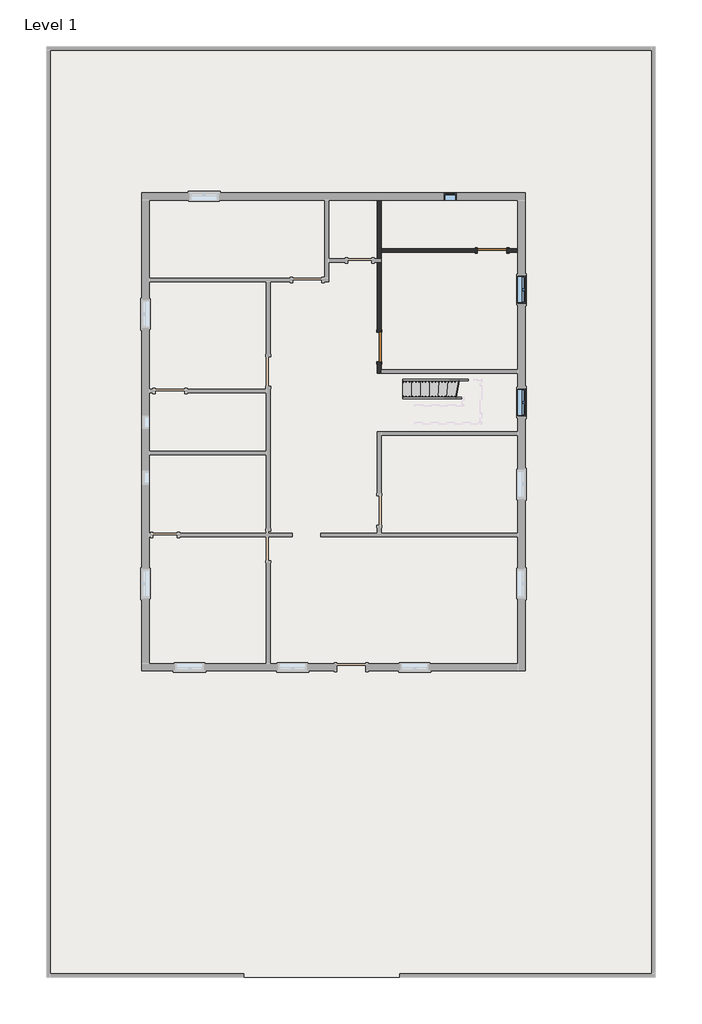
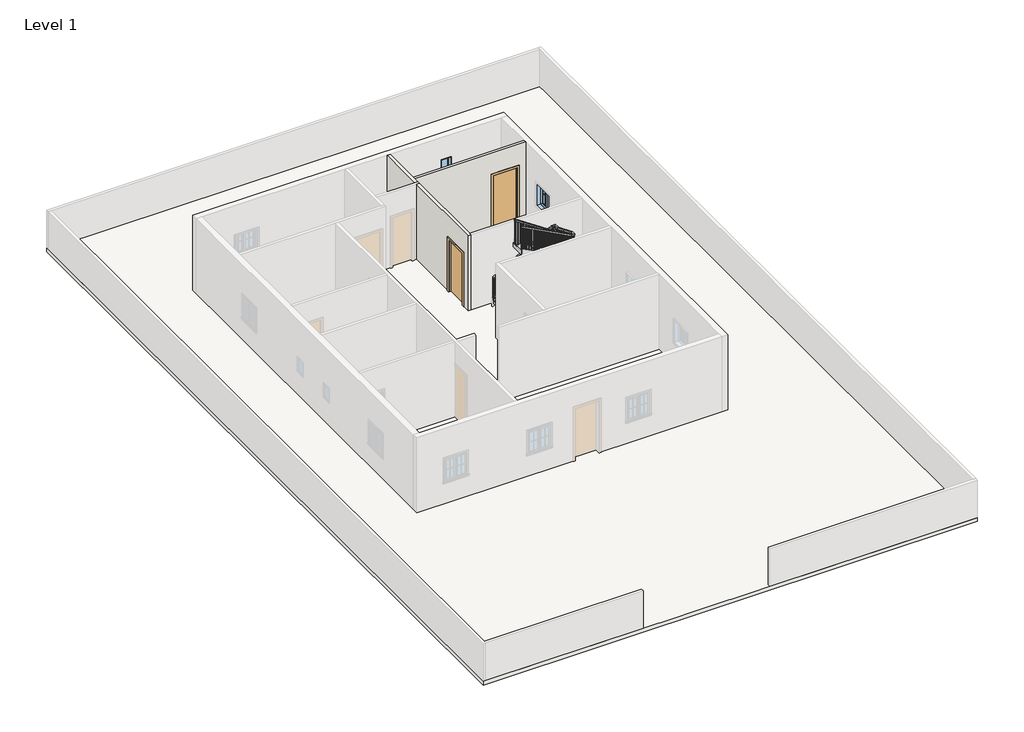
# One storey, part 2 of 3: 3 walls, 3 windows, 2 doors, 2 railings, 1 slab, 1 stair flight.
"""IFC4 building model written with IfcOpenShell, lengths in millimetres."""

from ifc_helpers import new_model, si_unit, frame, origin, place, context, project, spatial, polyline, outline, extrude, faceted_brep, transform, mapped, element, save
from components import door_e5f9f3c4, stair_flight_42adf773, window_373d1f99, window_339605e1

model = new_model("IFC4")

# Units and contexts
model_context = context("Model", 3, world=origin())
ifc_project = project(units=[si_unit("LENGTHUNIT", "METRE", prefix="MILLI")], contexts=[model_context])

# Site, building, storey
site = spatial("IfcSite", under=ifc_project)
building = spatial("IfcBuilding", under=site)
storey = spatial("IfcBuildingStorey", under=building, Name="Level 1", Elevation=0.0)

# Doors
placement = place(None, origin())
door_shape = door_e5f9f3c4(model_context)
element("IfcDoor", 1, ObjectType="Single-Flush : 36\" x 84\"", at=placement, inside=storey, context=model_context, shape_type="MappedRepresentation", body=[
    mapped(door_shape, transform((3624.6756993, 7272.227558, 0.0), x_axis=(1.0, 0.0, 0.0), y_axis=(0.0, 1.0, 0.0), z_axis=(0.0, 0.0, 1.0))),
])
element("IfcDoor", 2, ObjectType="Single-Flush : 36\" x 84\"", at=placement, inside=storey, context=model_context, shape_type="MappedRepresentation", body=[
    mapped(door_shape, transform((100.4256993, 4262.327558, 0.0), x_axis=(0.0, -1.0, 0.0), y_axis=(1.0, 0.0, 0.0), z_axis=(0.0, 0.0, 1.0))),
])

# Railings
element("IfcRailing", 3, ObjectType="Handrail - Rectangular", at=placement, inside=storey, context=model_context, shape_type="SolidModel", body=[
    faceted_brep([(838.4202681, 2744.677558, 1253.0666667), (838.4202681, 2744.677558, 1192.7442501), (838.4202681, 2693.877558, 1192.7442501), (838.4202681, 2693.877558, 1253.0666667), (2663.2073911, 2744.677558, 2421.5510761), (2714.0073911, 2744.677558, 2393.7579377), (2714.0073911, 2693.877558, 2393.7579377), (2663.2073911, 2693.877558, 2421.5510761), (2663.2073911, 2744.677558, 2633.8070819), (2714.0073911, 2744.677558, 2583.0070819), (2714.0073911, 2693.877558, 2583.0070819), (2663.2073911, 2693.877558, 2633.8070819), (2790.2073911, 2744.677558, 2633.8070819), (2790.2073911, 2744.677558, 2583.0070819), (2739.4073911, 2693.877558, 2583.0070819), (2739.4073911, 2693.877558, 2633.8070819), (2790.2073911, 2617.677558, 2633.8070819), (2790.2073911, 2595.5706127, 2583.0070819), (2739.4073911, 2595.5706127, 2583.0070819), (2739.4073911, 2617.677558, 2633.8070819), (2790.2073911, 2490.677558, 2770.1650362), (2790.2073911, 2439.877558, 2750.1723294), (2739.4073911, 2439.877558, 2750.1723294), (2739.4073911, 2490.677558, 2770.1650362), (2790.2073911, 2490.677558, 2985.7137911), (2790.2073911, 2439.877558, 2934.9137911), (2739.4073911, 2439.877558, 2934.9137911), (2739.4073911, 2490.677558, 2985.7137911), (2790.2073911, 2363.677558, 2985.7137911), (2790.2073911, 2363.677558, 2934.9137911), (2739.4073911, 2414.477558, 2934.9137911), (2739.4073911, 2414.477558, 2985.7137911), (2663.2073911, 2363.677558, 2985.7137911), (2647.7076469, 2363.677558, 2934.9137911), (2647.7076469, 2414.477558, 2934.9137911), (2663.2073911, 2414.477558, 2985.7137911), (1211.6756993, 2363.677558, 3962.4), (1211.6756993, 2414.477558, 3962.4), (1211.6756993, 2414.477558, 3901.1707504), (1211.6756993, 2363.677558, 3901.1707504)], [[[0, 1, 2, 3]], [[1, 0, 4, 5]], [[2, 1, 5, 6]], [[3, 2, 6, 7]], [[0, 3, 7, 4]], [[5, 4, 8, 9]], [[6, 5, 9, 10]], [[7, 6, 10, 11]], [[4, 7, 11, 8]], [[9, 8, 12, 13]], [[10, 9, 13, 14]], [[11, 10, 14, 15]], [[8, 11, 15, 12]], [[13, 12, 16, 17]], [[14, 13, 17, 18]], [[15, 14, 18, 19]], [[12, 15, 19, 16]], [[17, 16, 20, 21]], [[18, 17, 21, 22]], [[19, 18, 22, 23]], [[16, 19, 23, 20]], [[21, 20, 24, 25]], [[22, 21, 25, 26]], [[23, 22, 26, 27]], [[20, 23, 27, 24]], [[25, 24, 28, 29]], [[26, 25, 29, 30]], [[27, 26, 30, 31]], [[24, 27, 31, 28]], [[29, 28, 32, 33]], [[30, 29, 33, 34]], [[31, 30, 34, 35]], [[28, 31, 35, 32]], [[36, 37, 38, 39]], [[33, 32, 36, 39]], [[34, 33, 39, 38]], [[35, 34, 38, 37]], [[32, 35, 37, 36]]]),
    extrude(outline(polyline([(3875.1599798, 1250.3323911), (3887.9780756, 1231.2823911), (2878.6666667, 1231.2823911), (2878.6666667, 1250.3323911), (3875.1599798, 1250.3323911)])), frame((0.0, 2379.552558, 0.0), z_axis=(0.0, 1.0, 0.0), x_axis=(0.0, 0.0, 1.0)), (0.0, 0.0, 1.0), 19.05),
    extrude(outline(polyline([(3806.7968022, 1351.9323911), (3819.614898, 1332.8823911), (2878.6666667, 1332.8823911), (2878.6666667, 1351.9323911), (3806.7968022, 1351.9323911)])), frame((0.0, 2379.552558, 0.0), z_axis=(0.0, 1.0, 0.0), x_axis=(0.0, 0.0, 1.0)), (0.0, 0.0, 1.0), 19.05),
    extrude(outline(polyline([(3738.4336246, 1453.5323911), (3751.2517204, 1434.4823911), (2878.6666667, 1434.4823911), (2878.6666667, 1453.5323911), (3738.4336246, 1453.5323911)])), frame((0.0, 2379.552558, 0.0), z_axis=(0.0, 1.0, 0.0), x_axis=(0.0, 0.0, 1.0)), (0.0, 0.0, 1.0), 19.05),
    extrude(outline(polyline([(3670.070447, 1555.1323911), (3682.8885428, 1536.0823911), (2709.3333333, 1536.0823911), (2709.3333333, 1555.1323911), (3670.070447, 1555.1323911)])), frame((0.0, 2379.552558, 0.0), z_axis=(0.0, 1.0, 0.0), x_axis=(0.0, 0.0, 1.0)), (0.0, 0.0, 1.0), 19.05),
    extrude(outline(polyline([(3601.7072694, 1656.7323911), (3614.5253652, 1637.6823911), (2709.3333333, 1637.6823911), (2709.3333333, 1656.7323911), (3601.7072694, 1656.7323911)])), frame((0.0, 2379.552558, 0.0), z_axis=(0.0, 1.0, 0.0), x_axis=(0.0, 0.0, 1.0)), (0.0, 0.0, 1.0), 19.05),
    extrude(outline(polyline([(3533.3440918, 1758.3323911), (3546.1621876, 1739.2823911), (2709.3333333, 1739.2823911), (2709.3333333, 1758.3323911), (3533.3440918, 1758.3323911)])), frame((0.0, 2379.552558, 0.0), z_axis=(0.0, 1.0, 0.0), x_axis=(0.0, 0.0, 1.0)), (0.0, 0.0, 1.0), 19.05),
    extrude(outline(polyline([(3464.9809143, 1859.9323911), (3477.7990101, 1840.8823911), (2540.0, 1840.8823911), (2540.0, 1859.9323911), (3464.9809143, 1859.9323911)])), frame((0.0, 2379.552558, 0.0), z_axis=(0.0, 1.0, 0.0), x_axis=(0.0, 0.0, 1.0)), (0.0, 0.0, 1.0), 19.05),
    extrude(outline(polyline([(3396.6177367, 1961.5323911), (3409.4358325, 1942.4823911), (2540.0, 1942.4823911), (2540.0, 1961.5323911), (3396.6177367, 1961.5323911)])), frame((0.0, 2379.552558, 0.0), z_axis=(0.0, 1.0, 0.0), x_axis=(0.0, 0.0, 1.0)), (0.0, 0.0, 1.0), 19.05),
    extrude(outline(polyline([(3328.2545591, 2063.1323911), (3341.0726549, 2044.0823911), (2370.6666667, 2044.0823911), (2370.6666667, 2063.1323911), (3328.2545591, 2063.1323911)])), frame((0.0, 2379.552558, 0.0), z_axis=(0.0, 1.0, 0.0), x_axis=(0.0, 0.0, 1.0)), (0.0, 0.0, 1.0), 19.05),
    extrude(outline(polyline([(3259.8913815, 2164.7323911), (3272.7094773, 2145.6823911), (2370.6666667, 2145.6823911), (2370.6666667, 2164.7323911), (3259.8913815, 2164.7323911)])), frame((0.0, 2379.552558, 0.0), z_axis=(0.0, 1.0, 0.0), x_axis=(0.0, 0.0, 1.0)), (0.0, 0.0, 1.0), 19.05),
    extrude(outline(polyline([(3191.5282039, 2266.3323911), (3204.3462997, 2247.2823911), (2370.6666667, 2247.2823911), (2370.6666667, 2266.3323911), (3191.5282039, 2266.3323911)])), frame((0.0, 2379.552558, 0.0), z_axis=(0.0, 1.0, 0.0), x_axis=(0.0, 0.0, 1.0)), (0.0, 0.0, 1.0), 19.05),
    extrude(outline(polyline([(3123.1650263, 2367.9323911), (3135.9831221, 2348.8823911), (2201.3333333, 2348.8823911), (2201.3333333, 2367.9323911), (3123.1650263, 2367.9323911)])), frame((0.0, 2379.552558, 0.0), z_axis=(0.0, 1.0, 0.0), x_axis=(0.0, 0.0, 1.0)), (0.0, 0.0, 1.0), 19.05),
    extrude(outline(polyline([(3054.8018487, 2469.5323911), (3067.6199445, 2450.4823911), (2201.3333333, 2450.4823911), (2201.3333333, 2469.5323911), (3054.8018487, 2469.5323911)])), frame((0.0, 2379.552558, 0.0), z_axis=(0.0, 1.0, 0.0), x_axis=(0.0, 0.0, 1.0)), (0.0, 0.0, 1.0), 19.05),
    extrude(outline(polyline([(2986.4386712, 2571.1323911), (2999.256767, 2552.0823911), (2032.0, 2552.0823911), (2032.0, 2571.1323911), (2986.4386712, 2571.1323911)])), frame((0.0, 2379.552558, 0.0), z_axis=(0.0, 1.0, 0.0), x_axis=(0.0, 0.0, 1.0)), (0.0, 0.0, 1.0), 19.05),
    extrude(outline(polyline([(2918.0754936, 2672.7323911), (2930.8935894, 2653.6823911), (2032.0, 2653.6823911), (2032.0, 2672.7323911), (2918.0754936, 2672.7323911)])), frame((0.0, 2379.552558, 0.0), z_axis=(0.0, 1.0, 0.0), x_axis=(0.0, 0.0, 1.0)), (0.0, 0.0, 1.0), 19.05),
    extrude(outline(polyline([(2755.2823911, 2424.002558), (2774.3323911, 2424.002558), (2774.3323911, 2404.952558), (2755.2823911, 2404.952558), (2755.2823911, 2424.002558)])), frame((0.0, 0.0, 1862.6666667), z_axis=(0.0, 0.0, 1.0), x_axis=(1.0, 0.0, 0.0)), (0.0, 0.0, 1.0), 1072.2471245),
    extrude(outline(polyline([(2506.552558, 2678.5844034), (2525.602558, 2658.1307103), (2525.602558, 1693.3333333), (2506.552558, 1693.3333333), (2506.552558, 2678.5844034)])), frame((2755.2823911, 0.0, 0.0), z_axis=(1.0, 0.0, 0.0), x_axis=(0.0, 1.0, 0.0)), (0.0, 0.0, 1.0), 19.05),
    extrude(outline(polyline([(2608.152558, 2569.49804), (2627.202558, 2549.0443468), (2627.202558, 1693.3333333), (2608.152558, 1693.3333333), (2608.152558, 2569.49804)])), frame((2755.2823911, 0.0, 0.0), z_axis=(1.0, 0.0, 0.0), x_axis=(0.0, 1.0, 0.0)), (0.0, 0.0, 1.0), 19.05),
    extrude(outline(polyline([(2657.6952681, 2709.752558), (2657.6952681, 2728.802558), (2676.7452681, 2728.802558), (2676.7452681, 2709.752558), (2657.6952681, 2709.752558)])), frame((0.0, 0.0, 1354.6666667), z_axis=(0.0, 0.0, 1.0), x_axis=(1.0, 0.0, 0.0)), (0.0, 0.0, 1.0), 1228.3404152),
    extrude(outline(polyline([(2304.8389489, 2575.1452681), (2292.6404695, 2556.0952681), (1354.6666667, 2556.0952681), (1354.6666667, 2575.1452681), (2304.8389489, 2575.1452681)])), frame((0.0, 2709.752558, 0.0), z_axis=(0.0, 1.0, 0.0), x_axis=(0.0, 0.0, 1.0)), (0.0, 0.0, 1.0), 19.05),
    extrude(outline(polyline([(2239.7803925, 2473.5452681), (2227.5819131, 2454.4952681), (1185.3333333, 2454.4952681), (1185.3333333, 2473.5452681), (2239.7803925, 2473.5452681)])), frame((0.0, 2709.752558, 0.0), z_axis=(0.0, 1.0, 0.0), x_axis=(0.0, 0.0, 1.0)), (0.0, 0.0, 1.0), 19.05),
    extrude(outline(polyline([(2174.721836, 2371.9452681), (2162.5233567, 2352.8952681), (1185.3333333, 2352.8952681), (1185.3333333, 2371.9452681), (2174.721836, 2371.9452681)])), frame((0.0, 2709.752558, 0.0), z_axis=(0.0, 1.0, 0.0), x_axis=(0.0, 0.0, 1.0)), (0.0, 0.0, 1.0), 19.05),
    extrude(outline(polyline([(2109.6632796, 2270.3452681), (2097.4648003, 2251.2952681), (1185.3333333, 2251.2952681), (1185.3333333, 2270.3452681), (2109.6632796, 2270.3452681)])), frame((0.0, 2709.752558, 0.0), z_axis=(0.0, 1.0, 0.0), x_axis=(0.0, 0.0, 1.0)), (0.0, 0.0, 1.0), 19.05),
    extrude(outline(polyline([(2044.6047232, 2168.7452681), (2032.4062439, 2149.6952681), (1016.0, 2149.6952681), (1016.0, 2168.7452681), (2044.6047232, 2168.7452681)])), frame((0.0, 2709.752558, 0.0), z_axis=(0.0, 1.0, 0.0), x_axis=(0.0, 0.0, 1.0)), (0.0, 0.0, 1.0), 19.05),
    extrude(outline(polyline([(1979.5461668, 2067.1452681), (1967.3476875, 2048.0952681), (1016.0, 2048.0952681), (1016.0, 2067.1452681), (1979.5461668, 2067.1452681)])), frame((0.0, 2709.752558, 0.0), z_axis=(0.0, 1.0, 0.0), x_axis=(0.0, 0.0, 1.0)), (0.0, 0.0, 1.0), 19.05),
    extrude(outline(polyline([(1914.4876104, 1965.5452681), (1902.289131, 1946.4952681), (1016.0, 1946.4952681), (1016.0, 1965.5452681), (1914.4876104, 1965.5452681)])), frame((0.0, 2709.752558, 0.0), z_axis=(0.0, 1.0, 0.0), x_axis=(0.0, 0.0, 1.0)), (0.0, 0.0, 1.0), 19.05),
    extrude(outline(polyline([(1849.4290539, 1863.9452681), (1837.2305746, 1844.8952681), (846.6666667, 1844.8952681), (846.6666667, 1863.9452681), (1849.4290539, 1863.9452681)])), frame((0.0, 2709.752558, 0.0), z_axis=(0.0, 1.0, 0.0), x_axis=(0.0, 0.0, 1.0)), (0.0, 0.0, 1.0), 19.05),
    extrude(outline(polyline([(1784.3704975, 1762.3452681), (1772.1720182, 1743.2952681), (846.6666667, 1743.2952681), (846.6666667, 1762.3452681), (1784.3704975, 1762.3452681)])), frame((0.0, 2709.752558, 0.0), z_axis=(0.0, 1.0, 0.0), x_axis=(0.0, 0.0, 1.0)), (0.0, 0.0, 1.0), 19.05),
    extrude(outline(polyline([(1719.3119411, 1660.7452681), (1707.1134618, 1641.6952681), (677.3333333, 1641.6952681), (677.3333333, 1660.7452681), (1719.3119411, 1660.7452681)])), frame((0.0, 2709.752558, 0.0), z_axis=(0.0, 1.0, 0.0), x_axis=(0.0, 0.0, 1.0)), (0.0, 0.0, 1.0), 19.05),
    extrude(outline(polyline([(1654.2533847, 1559.1452681), (1642.0549054, 1540.0952681), (677.3333333, 1540.0952681), (677.3333333, 1559.1452681), (1654.2533847, 1559.1452681)])), frame((0.0, 2709.752558, 0.0), z_axis=(0.0, 1.0, 0.0), x_axis=(0.0, 0.0, 1.0)), (0.0, 0.0, 1.0), 19.05),
    extrude(outline(polyline([(1589.1948283, 1457.5452681), (1576.9963489, 1438.4952681), (677.3333333, 1438.4952681), (677.3333333, 1457.5452681), (1589.1948283, 1457.5452681)])), frame((0.0, 2709.752558, 0.0), z_axis=(0.0, 1.0, 0.0), x_axis=(0.0, 0.0, 1.0)), (0.0, 0.0, 1.0), 19.05),
    extrude(outline(polyline([(1524.1362719, 1355.9452681), (1511.9377925, 1336.8952681), (508.0, 1336.8952681), (508.0, 1355.9452681), (1524.1362719, 1355.9452681)])), frame((0.0, 2709.752558, 0.0), z_axis=(0.0, 1.0, 0.0), x_axis=(0.0, 0.0, 1.0)), (0.0, 0.0, 1.0), 19.05),
    extrude(outline(polyline([(1459.0777154, 1254.3452681), (1446.8792361, 1235.2952681), (508.0, 1235.2952681), (508.0, 1254.3452681), (1459.0777154, 1254.3452681)])), frame((0.0, 2709.752558, 0.0), z_axis=(0.0, 1.0, 0.0), x_axis=(0.0, 0.0, 1.0)), (0.0, 0.0, 1.0), 19.05),
    extrude(outline(polyline([(1394.019159, 1152.7452681), (1381.8206797, 1133.6952681), (508.0, 1133.6952681), (508.0, 1152.7452681), (1394.019159, 1152.7452681)])), frame((0.0, 2709.752558, 0.0), z_axis=(0.0, 1.0, 0.0), x_axis=(0.0, 0.0, 1.0)), (0.0, 0.0, 1.0), 19.05),
    extrude(outline(polyline([(1328.9606026, 1051.1452681), (1316.7621233, 1032.0952681), (338.6666667, 1032.0952681), (338.6666667, 1051.1452681), (1328.9606026, 1051.1452681)])), frame((0.0, 2709.752558, 0.0), z_axis=(0.0, 1.0, 0.0), x_axis=(0.0, 0.0, 1.0)), (0.0, 0.0, 1.0), 19.05),
    extrude(outline(polyline([(1263.9020462, 949.5452681), (1251.7035669, 930.4952681), (338.6666667, 930.4952681), (338.6666667, 949.5452681), (1263.9020462, 949.5452681)])), frame((0.0, 2709.752558, 0.0), z_axis=(0.0, 1.0, 0.0), x_axis=(0.0, 0.0, 1.0)), (0.0, 0.0, 1.0), 19.05),
    extrude(outline(polyline([(2755.2823911, 2398.602558), (2774.3323911, 2398.602558), (2774.3323911, 2379.552558), (2755.2823911, 2379.552558), (2755.2823911, 2398.602558)])), frame((0.0, 0.0, 1862.6666667), z_axis=(0.0, 0.0, 1.0), x_axis=(1.0, 0.0, 0.0)), (0.0, 0.0, 1.0), 1072.2471245),
    extrude(outline(polyline([(2755.2823911, 2709.752558), (2755.2823911, 2728.802558), (2774.3323911, 2728.802558), (2774.3323911, 2709.752558), (2755.2823911, 2709.752558)])), frame((0.0, 0.0, 1524.0), z_axis=(0.0, 0.0, 1.0), x_axis=(1.0, 0.0, 0.0)), (0.0, 0.0, 1.0), 1059.0070819),
    extrude(outline(polyline([(3888.3526546, 1230.7256993), (3901.1707504, 1211.6756993), (2878.6666667, 1211.6756993), (2878.6666667, 1230.7256993), (3888.3526546, 1230.7256993)])), frame((0.0, 2379.552558, 0.0), z_axis=(0.0, 1.0, 0.0), x_axis=(0.0, 0.0, 1.0)), (0.0, 0.0, 1.0), 19.05),
    extrude(outline(polyline([(1204.9427294, 857.4702681), (1192.7442501, 838.4202681), (338.6666667, 838.4202681), (338.6666667, 857.4702681), (1204.9427294, 857.4702681)])), frame((0.0, 2709.752558, 0.0), z_axis=(0.0, 1.0, 0.0), x_axis=(0.0, 0.0, 1.0)), (0.0, 0.0, 1.0), 19.05),
])
element("IfcRailing", 4, ObjectType="Handrail - Rectangular", at=placement, inside=storey, context=model_context, shape_type="SolidModel", body=[
    faceted_brep([(838.4202681, 3202.4524989, 1253.0666667), (838.4202681, 3202.4524989, 1194.4953096), (838.4202681, 3151.6524989, 1194.4953096), (838.4202681, 3151.6524989, 1253.0666667), (3089.9785641, 3202.4524989, 2545.2368493), (3103.5198636, 3202.4524989, 2494.4368493), (3103.5198636, 3151.6524989, 2494.4368493), (3089.9785641, 3151.6524989, 2545.2368493), (3247.982332, 3202.4524989, 2545.2368493), (3247.982332, 3202.4524989, 2494.4368493), (3197.182332, 3151.6524989, 2494.4368493), (3197.182332, 3151.6524989, 2545.2368493), (3247.982332, 2995.1725832, 2545.2368493), (3247.982332, 2984.9732412, 2494.4368493), (3197.182332, 2984.9732412, 2494.4368493), (3197.182332, 2995.1725832, 2545.2368493), (3247.982332, 2050.6126885, 2940.4552365), (3247.982332, 2040.4133465, 2889.6552365), (3197.182332, 2040.4133465, 2889.6552365), (3197.182332, 2050.6126885, 2940.4552365), (3247.982332, 1905.9026171, 2940.4552365), (3247.982332, 1905.9026171, 2889.6552365), (3197.182332, 1956.7026171, 2889.6552365), (3197.182332, 1956.7026171, 2940.4552365), (3128.9262072, 1905.9026171, 2940.4552365), (3116.2326609, 1905.9026171, 2889.6552365), (3116.2326609, 1956.7026171, 2889.6552365), (3128.9262072, 1956.7026171, 2940.4552365), (1211.6756993, 1905.9026171, 3962.4), (1211.6756993, 1956.7026171, 3962.4), (1211.6756993, 1956.7026171, 3904.8340072), (1211.6756993, 1905.9026171, 3904.8340072)], [[[0, 1, 2, 3]], [[1, 0, 4, 5]], [[2, 1, 5, 6]], [[3, 2, 6, 7]], [[0, 3, 7, 4]], [[5, 4, 8, 9]], [[6, 5, 9, 10]], [[7, 6, 10, 11]], [[4, 7, 11, 8]], [[9, 8, 12, 13]], [[10, 9, 13, 14]], [[11, 10, 14, 15]], [[8, 11, 15, 12]], [[13, 12, 16, 17]], [[14, 13, 17, 18]], [[15, 14, 18, 19]], [[12, 15, 19, 16]], [[17, 16, 20, 21]], [[18, 17, 21, 22]], [[19, 18, 22, 23]], [[16, 19, 23, 20]], [[21, 20, 24, 25]], [[22, 21, 25, 26]], [[23, 22, 26, 27]], [[20, 23, 27, 24]], [[28, 29, 30, 31]], [[25, 24, 28, 31]], [[26, 25, 31, 30]], [[27, 26, 30, 29]], [[24, 27, 29, 28]]]),
    extrude(outline(polyline([(3866.9989368, 1282.657332), (2878.6666667, 1282.657332), (2878.6666667, 1301.707332), (3856.8447876, 1301.707332), (3866.9989368, 1282.657332)])), frame((0.0, 1921.7776171, 0.0), z_axis=(0.0, 1.0, 0.0), x_axis=(0.0, 0.0, 1.0)), (0.0, 0.0, 1.0), 19.05),
    extrude(outline(polyline([(3812.8434743, 1384.257332), (2878.6666667, 1384.257332), (2878.6666667, 1403.307332), (3802.6893251, 1403.307332), (3812.8434743, 1384.257332)])), frame((0.0, 1921.7776171, 0.0), z_axis=(0.0, 1.0, 0.0), x_axis=(0.0, 0.0, 1.0)), (0.0, 0.0, 1.0), 19.05),
    extrude(outline(polyline([(3758.6880118, 1485.857332), (2709.3333333, 1485.857332), (2709.3333333, 1504.907332), (3748.5338626, 1504.907332), (3758.6880118, 1485.857332)])), frame((0.0, 1921.7776171, 0.0), z_axis=(0.0, 1.0, 0.0), x_axis=(0.0, 0.0, 1.0)), (0.0, 0.0, 1.0), 19.05),
    extrude(outline(polyline([(3704.5325493, 1587.457332), (2709.3333333, 1587.457332), (2709.3333333, 1606.507332), (3694.3784001, 1606.507332), (3704.5325493, 1587.457332)])), frame((0.0, 1921.7776171, 0.0), z_axis=(0.0, 1.0, 0.0), x_axis=(0.0, 0.0, 1.0)), (0.0, 0.0, 1.0), 19.05),
    extrude(outline(polyline([(3650.3770868, 1689.057332), (2709.3333333, 1689.057332), (2709.3333333, 1708.107332), (3640.2229376, 1708.107332), (3650.3770868, 1689.057332)])), frame((0.0, 1921.7776171, 0.0), z_axis=(0.0, 1.0, 0.0), x_axis=(0.0, 0.0, 1.0)), (0.0, 0.0, 1.0), 19.05),
    extrude(outline(polyline([(3596.2216243, 1790.657332), (2540.0, 1790.657332), (2540.0, 1809.707332), (3586.0674751, 1809.707332), (3596.2216243, 1790.657332)])), frame((0.0, 1921.7776171, 0.0), z_axis=(0.0, 1.0, 0.0), x_axis=(0.0, 0.0, 1.0)), (0.0, 0.0, 1.0), 19.05),
    extrude(outline(polyline([(3542.0661618, 1892.257332), (2540.0, 1892.257332), (2540.0, 1911.307332), (3531.9120126, 1911.307332), (3542.0661618, 1892.257332)])), frame((0.0, 1921.7776171, 0.0), z_axis=(0.0, 1.0, 0.0), x_axis=(0.0, 0.0, 1.0)), (0.0, 0.0, 1.0), 19.05),
    extrude(outline(polyline([(3487.9106993, 1993.857332), (2540.0, 1993.857332), (2540.0, 2012.907332), (3477.7565501, 2012.907332), (3487.9106993, 1993.857332)])), frame((0.0, 1921.7776171, 0.0), z_axis=(0.0, 1.0, 0.0), x_axis=(0.0, 0.0, 1.0)), (0.0, 0.0, 1.0), 19.05),
    extrude(outline(polyline([(3433.7552369, 2095.457332), (2370.6666667, 2095.457332), (2370.6666667, 2114.507332), (3423.6010876, 2114.507332), (3433.7552369, 2095.457332)])), frame((0.0, 1921.7776171, 0.0), z_axis=(0.0, 1.0, 0.0), x_axis=(0.0, 0.0, 1.0)), (0.0, 0.0, 1.0), 19.05),
    extrude(outline(polyline([(3379.5997744, 2197.057332), (2370.6666667, 2197.057332), (2370.6666667, 2216.107332), (3369.4456251, 2216.107332), (3379.5997744, 2197.057332)])), frame((0.0, 1921.7776171, 0.0), z_axis=(0.0, 1.0, 0.0), x_axis=(0.0, 0.0, 1.0)), (0.0, 0.0, 1.0), 19.05),
    extrude(outline(polyline([(3325.4443119, 2298.657332), (2370.6666667, 2298.657332), (2370.6666667, 2317.707332), (3315.2901626, 2317.707332), (3325.4443119, 2298.657332)])), frame((0.0, 1921.7776171, 0.0), z_axis=(0.0, 1.0, 0.0), x_axis=(0.0, 0.0, 1.0)), (0.0, 0.0, 1.0), 19.05),
    extrude(outline(polyline([(3271.2888494, 2400.257332), (2201.3333333, 2400.257332), (2201.3333333, 2419.307332), (3261.1347002, 2419.307332), (3271.2888494, 2400.257332)])), frame((0.0, 1921.7776171, 0.0), z_axis=(0.0, 1.0, 0.0), x_axis=(0.0, 0.0, 1.0)), (0.0, 0.0, 1.0), 19.05),
    extrude(outline(polyline([(3217.1333869, 2501.857332), (2201.3333333, 2501.857332), (2201.3333333, 2520.907332), (3206.9792377, 2520.907332), (3217.1333869, 2501.857332)])), frame((0.0, 1921.7776171, 0.0), z_axis=(0.0, 1.0, 0.0), x_axis=(0.0, 0.0, 1.0)), (0.0, 0.0, 1.0), 19.05),
    extrude(outline(polyline([(3162.9779244, 2603.457332), (2201.3333333, 2603.457332), (2201.3333333, 2622.507332), (3152.8237752, 2622.507332), (3162.9779244, 2603.457332)])), frame((0.0, 1921.7776171, 0.0), z_axis=(0.0, 1.0, 0.0), x_axis=(0.0, 0.0, 1.0)), (0.0, 0.0, 1.0), 19.05),
    extrude(outline(polyline([(3108.8224619, 2705.057332), (2032.0, 2705.057332), (2032.0, 2724.107332), (3098.6683127, 2724.107332), (3108.8224619, 2705.057332)])), frame((0.0, 1921.7776171, 0.0), z_axis=(0.0, 1.0, 0.0), x_axis=(0.0, 0.0, 1.0)), (0.0, 0.0, 1.0), 19.05),
    extrude(outline(polyline([(3054.6669994, 2806.657332), (2032.0, 2806.657332), (2032.0, 2825.707332), (3044.5128502, 2825.707332), (3054.6669994, 2806.657332)])), frame((0.0, 1921.7776171, 0.0), z_axis=(0.0, 1.0, 0.0), x_axis=(0.0, 0.0, 1.0)), (0.0, 0.0, 1.0), 19.05),
    extrude(outline(polyline([(3000.5115369, 2908.257332), (2032.0, 2908.257332), (2032.0, 2927.307332), (2990.3573877, 2927.307332), (3000.5115369, 2908.257332)])), frame((0.0, 1921.7776171, 0.0), z_axis=(0.0, 1.0, 0.0), x_axis=(0.0, 0.0, 1.0)), (0.0, 0.0, 1.0), 19.05),
    extrude(outline(polyline([(2946.3560744, 3009.857332), (2032.0, 3009.857332), (2032.0, 3028.907332), (2936.2019252, 3028.907332), (2946.3560744, 3009.857332)])), frame((0.0, 1921.7776171, 0.0), z_axis=(0.0, 1.0, 0.0), x_axis=(0.0, 0.0, 1.0)), (0.0, 0.0, 1.0), 19.05),
    extrude(outline(polyline([(2892.2006119, 3111.457332), (1862.6666667, 3111.457332), (1862.6666667, 3130.507332), (2882.0464627, 3130.507332), (2892.2006119, 3111.457332)])), frame((0.0, 1921.7776171, 0.0), z_axis=(0.0, 1.0, 0.0), x_axis=(0.0, 0.0, 1.0)), (0.0, 0.0, 1.0), 19.05),
    extrude(outline(polyline([(3232.107332, 1967.3774989), (3232.107332, 1948.3274989), (3213.057332, 1948.3274989), (3213.057332, 1967.3774989), (3232.107332, 1967.3774989)])), frame((0.0, 0.0, 1862.6666667), z_axis=(0.0, 0.0, 1.0), x_axis=(1.0, 0.0, 0.0)), (0.0, 0.0, 1.0), 1026.9885698),
    extrude(outline(polyline([(2068.9774989, 2877.7035558), (2068.9774989, 1862.6666667), (2049.9274989, 1862.6666667), (2049.9274989, 2885.6743688), (2068.9774989, 2877.7035558)])), frame((3213.057332, 0.0, 0.0), z_axis=(1.0, 0.0, 0.0), x_axis=(0.0, 1.0, 0.0)), (0.0, 0.0, 1.0), 19.05),
    extrude(outline(polyline([(2170.5774989, 2835.1925532), (2170.5774989, 1862.6666667), (2151.5274989, 1862.6666667), (2151.5274989, 2843.1633662), (2170.5774989, 2835.1925532)])), frame((3213.057332, 0.0, 0.0), z_axis=(1.0, 0.0, 0.0), x_axis=(0.0, 1.0, 0.0)), (0.0, 0.0, 1.0), 19.05),
    extrude(outline(polyline([(2272.1774989, 2792.6815506), (2272.1774989, 1862.6666667), (2253.1274989, 1862.6666667), (2253.1274989, 2800.6523636), (2272.1774989, 2792.6815506)])), frame((3213.057332, 0.0, 0.0), z_axis=(1.0, 0.0, 0.0), x_axis=(0.0, 1.0, 0.0)), (0.0, 0.0, 1.0), 19.05),
    extrude(outline(polyline([(2373.7774989, 2750.170548), (2373.7774989, 1862.6666667), (2354.7274989, 1862.6666667), (2354.7274989, 2758.141361), (2373.7774989, 2750.170548)])), frame((3213.057332, 0.0, 0.0), z_axis=(1.0, 0.0, 0.0), x_axis=(0.0, 1.0, 0.0)), (0.0, 0.0, 1.0), 19.05),
    extrude(outline(polyline([(2475.3774989, 2707.6595454), (2475.3774989, 1693.3333333), (2456.3274989, 1693.3333333), (2456.3274989, 2715.6303584), (2475.3774989, 2707.6595454)])), frame((3213.057332, 0.0, 0.0), z_axis=(1.0, 0.0, 0.0), x_axis=(0.0, 1.0, 0.0)), (0.0, 0.0, 1.0), 19.05),
    extrude(outline(polyline([(2576.9774989, 2665.1485428), (2576.9774989, 1693.3333333), (2557.9274989, 1693.3333333), (2557.9274989, 2673.1193558), (2576.9774989, 2665.1485428)])), frame((3213.057332, 0.0, 0.0), z_axis=(1.0, 0.0, 0.0), x_axis=(0.0, 1.0, 0.0)), (0.0, 0.0, 1.0), 19.05),
    extrude(outline(polyline([(2678.5774989, 2622.6375402), (2678.5774989, 1693.3333333), (2659.5274989, 1693.3333333), (2659.5274989, 2630.6083532), (2678.5774989, 2622.6375402)])), frame((3213.057332, 0.0, 0.0), z_axis=(1.0, 0.0, 0.0), x_axis=(0.0, 1.0, 0.0)), (0.0, 0.0, 1.0), 19.05),
    extrude(outline(polyline([(2780.1774989, 2580.1265376), (2780.1774989, 1693.3333333), (2761.1274989, 1693.3333333), (2761.1274989, 2588.0973506), (2780.1774989, 2580.1265376)])), frame((3213.057332, 0.0, 0.0), z_axis=(1.0, 0.0, 0.0), x_axis=(0.0, 1.0, 0.0)), (0.0, 0.0, 1.0), 19.05),
    extrude(outline(polyline([(2881.7774989, 2537.615535), (2881.7774989, 1524.0), (2862.7274989, 1524.0), (2862.7274989, 2545.586348), (2881.7774989, 2537.615535)])), frame((3213.057332, 0.0, 0.0), z_axis=(1.0, 0.0, 0.0), x_axis=(0.0, 1.0, 0.0)), (0.0, 0.0, 1.0), 19.05),
    extrude(outline(polyline([(2983.3774989, 2495.1045324), (2983.3774989, 1524.0), (2964.3274989, 1524.0), (2964.3274989, 2503.0753454), (2983.3774989, 2495.1045324)])), frame((3213.057332, 0.0, 0.0), z_axis=(1.0, 0.0, 0.0), x_axis=(0.0, 1.0, 0.0)), (0.0, 0.0, 1.0), 19.05),
    extrude(outline(polyline([(3232.107332, 3084.9774989), (3232.107332, 3065.9274989), (3213.057332, 3065.9274989), (3213.057332, 3084.9774989), (3232.107332, 3084.9774989)])), frame((0.0, 0.0, 1524.0), z_axis=(0.0, 0.0, 1.0), x_axis=(1.0, 0.0, 0.0)), (0.0, 0.0, 1.0), 970.4368493),
    extrude(outline(polyline([(3165.6952681, 3186.5774989), (3184.7452681, 3186.5774989), (3184.7452681, 3167.5274989), (3165.6952681, 3167.5274989), (3165.6952681, 3186.5774989)])), frame((0.0, 0.0, 1524.0), z_axis=(0.0, 0.0, 1.0), x_axis=(1.0, 0.0, 0.0)), (0.0, 0.0, 1.0), 970.4368493),
    extrude(outline(polyline([(2471.8110585, 3064.0952681), (1524.0, 3064.0952681), (1524.0, 3083.1452681), (2482.743861, 3083.1452681), (2471.8110585, 3064.0952681)])), frame((0.0, 3167.5274989, 0.0), z_axis=(0.0, 1.0, 0.0), x_axis=(0.0, 0.0, 1.0)), (0.0, 0.0, 1.0), 19.05),
    extrude(outline(polyline([(2413.502779, 2962.4952681), (1524.0, 2962.4952681), (1524.0, 2981.5452681), (2424.4355814, 2981.5452681), (2413.502779, 2962.4952681)])), frame((0.0, 3167.5274989, 0.0), z_axis=(0.0, 1.0, 0.0), x_axis=(0.0, 0.0, 1.0)), (0.0, 0.0, 1.0), 19.05),
    extrude(outline(polyline([(2355.1944994, 2860.8952681), (1354.6666667, 2860.8952681), (1354.6666667, 2879.9452681), (2366.1273019, 2879.9452681), (2355.1944994, 2860.8952681)])), frame((0.0, 3167.5274989, 0.0), z_axis=(0.0, 1.0, 0.0), x_axis=(0.0, 0.0, 1.0)), (0.0, 0.0, 1.0), 19.05),
    extrude(outline(polyline([(2296.8862199, 2759.2952681), (1354.6666667, 2759.2952681), (1354.6666667, 2778.3452681), (2307.8190223, 2778.3452681), (2296.8862199, 2759.2952681)])), frame((0.0, 3167.5274989, 0.0), z_axis=(0.0, 1.0, 0.0), x_axis=(0.0, 0.0, 1.0)), (0.0, 0.0, 1.0), 19.05),
    extrude(outline(polyline([(2238.5779403, 2657.6952681), (1354.6666667, 2657.6952681), (1354.6666667, 2676.7452681), (2249.5107428, 2676.7452681), (2238.5779403, 2657.6952681)])), frame((0.0, 3167.5274989, 0.0), z_axis=(0.0, 1.0, 0.0), x_axis=(0.0, 0.0, 1.0)), (0.0, 0.0, 1.0), 19.05),
    extrude(outline(polyline([(2180.2696608, 2556.0952681), (1354.6666667, 2556.0952681), (1354.6666667, 2575.1452681), (2191.2024632, 2575.1452681), (2180.2696608, 2556.0952681)])), frame((0.0, 3167.5274989, 0.0), z_axis=(0.0, 1.0, 0.0), x_axis=(0.0, 0.0, 1.0)), (0.0, 0.0, 1.0), 19.05),
    extrude(outline(polyline([(2121.9613812, 2454.4952681), (1185.3333333, 2454.4952681), (1185.3333333, 2473.5452681), (2132.8941837, 2473.5452681), (2121.9613812, 2454.4952681)])), frame((0.0, 3167.5274989, 0.0), z_axis=(0.0, 1.0, 0.0), x_axis=(0.0, 0.0, 1.0)), (0.0, 0.0, 1.0), 19.05),
    extrude(outline(polyline([(2063.6531017, 2352.8952681), (1185.3333333, 2352.8952681), (1185.3333333, 2371.9452681), (2074.5859041, 2371.9452681), (2063.6531017, 2352.8952681)])), frame((0.0, 3167.5274989, 0.0), z_axis=(0.0, 1.0, 0.0), x_axis=(0.0, 0.0, 1.0)), (0.0, 0.0, 1.0), 19.05),
    extrude(outline(polyline([(2005.3448221, 2251.2952681), (1185.3333333, 2251.2952681), (1185.3333333, 2270.3452681), (2016.2776245, 2270.3452681), (2005.3448221, 2251.2952681)])), frame((0.0, 3167.5274989, 0.0), z_axis=(0.0, 1.0, 0.0), x_axis=(0.0, 0.0, 1.0)), (0.0, 0.0, 1.0), 19.05),
    extrude(outline(polyline([(1947.0365426, 2149.6952681), (1016.0, 2149.6952681), (1016.0, 2168.7452681), (1957.969345, 2168.7452681), (1947.0365426, 2149.6952681)])), frame((0.0, 3167.5274989, 0.0), z_axis=(0.0, 1.0, 0.0), x_axis=(0.0, 0.0, 1.0)), (0.0, 0.0, 1.0), 19.05),
    extrude(outline(polyline([(1888.728263, 2048.0952681), (1016.0, 2048.0952681), (1016.0, 2067.1452681), (1899.6610654, 2067.1452681), (1888.728263, 2048.0952681)])), frame((0.0, 3167.5274989, 0.0), z_axis=(0.0, 1.0, 0.0), x_axis=(0.0, 0.0, 1.0)), (0.0, 0.0, 1.0), 19.05),
    extrude(outline(polyline([(1830.4199835, 1946.4952681), (846.6666667, 1946.4952681), (846.6666667, 1965.5452681), (1841.3527859, 1965.5452681), (1830.4199835, 1946.4952681)])), frame((0.0, 3167.5274989, 0.0), z_axis=(0.0, 1.0, 0.0), x_axis=(0.0, 0.0, 1.0)), (0.0, 0.0, 1.0), 19.05),
    extrude(outline(polyline([(1772.1117039, 1844.8952681), (846.6666667, 1844.8952681), (846.6666667, 1863.9452681), (1783.0445063, 1863.9452681), (1772.1117039, 1844.8952681)])), frame((0.0, 3167.5274989, 0.0), z_axis=(0.0, 1.0, 0.0), x_axis=(0.0, 0.0, 1.0)), (0.0, 0.0, 1.0), 19.05),
    extrude(outline(polyline([(1713.8034244, 1743.2952681), (846.6666667, 1743.2952681), (846.6666667, 1762.3452681), (1724.7362268, 1762.3452681), (1713.8034244, 1743.2952681)])), frame((0.0, 3167.5274989, 0.0), z_axis=(0.0, 1.0, 0.0), x_axis=(0.0, 0.0, 1.0)), (0.0, 0.0, 1.0), 19.05),
    extrude(outline(polyline([(1655.4951448, 1641.6952681), (677.3333333, 1641.6952681), (677.3333333, 1660.7452681), (1666.4279472, 1660.7452681), (1655.4951448, 1641.6952681)])), frame((0.0, 3167.5274989, 0.0), z_axis=(0.0, 1.0, 0.0), x_axis=(0.0, 0.0, 1.0)), (0.0, 0.0, 1.0), 19.05),
    extrude(outline(polyline([(1597.1868653, 1540.0952681), (677.3333333, 1540.0952681), (677.3333333, 1559.1452681), (1608.1196677, 1559.1452681), (1597.1868653, 1540.0952681)])), frame((0.0, 3167.5274989, 0.0), z_axis=(0.0, 1.0, 0.0), x_axis=(0.0, 0.0, 1.0)), (0.0, 0.0, 1.0), 19.05),
    extrude(outline(polyline([(1538.8785857, 1438.4952681), (677.3333333, 1438.4952681), (677.3333333, 1457.5452681), (1549.8113881, 1457.5452681), (1538.8785857, 1438.4952681)])), frame((0.0, 3167.5274989, 0.0), z_axis=(0.0, 1.0, 0.0), x_axis=(0.0, 0.0, 1.0)), (0.0, 0.0, 1.0), 19.05),
    extrude(outline(polyline([(1480.5703062, 1336.8952681), (508.0, 1336.8952681), (508.0, 1355.9452681), (1491.5031086, 1355.9452681), (1480.5703062, 1336.8952681)])), frame((0.0, 3167.5274989, 0.0), z_axis=(0.0, 1.0, 0.0), x_axis=(0.0, 0.0, 1.0)), (0.0, 0.0, 1.0), 19.05),
    extrude(outline(polyline([(1422.2620266, 1235.2952681), (508.0, 1235.2952681), (508.0, 1254.3452681), (1433.194829, 1254.3452681), (1422.2620266, 1235.2952681)])), frame((0.0, 3167.5274989, 0.0), z_axis=(0.0, 1.0, 0.0), x_axis=(0.0, 0.0, 1.0)), (0.0, 0.0, 1.0), 19.05),
    extrude(outline(polyline([(1363.828643, 1133.6952681), (508.0, 1133.6952681), (508.0, 1152.7452681), (1374.7614454, 1152.7452681), (1363.828643, 1133.6952681)])), frame((0.0, 3167.5274989, 0.0), z_axis=(0.0, 1.0, 0.0), x_axis=(0.0, 0.0, 1.0)), (0.0, 0.0, 1.0), 19.05),
    extrude(outline(polyline([(1305.6454675, 1032.0952681), (338.6666667, 1032.0952681), (338.6666667, 1051.1452681), (1316.5782699, 1051.1452681), (1305.6454675, 1032.0952681)])), frame((0.0, 3167.5274989, 0.0), z_axis=(0.0, 1.0, 0.0), x_axis=(0.0, 0.0, 1.0)), (0.0, 0.0, 1.0), 19.05),
    extrude(outline(polyline([(1247.337188, 930.4952681), (338.6666667, 930.4952681), (338.6666667, 949.5452681), (1258.2699904, 949.5452681), (1247.337188, 930.4952681)])), frame((0.0, 3167.5274989, 0.0), z_axis=(0.0, 1.0, 0.0), x_axis=(0.0, 0.0, 1.0)), (0.0, 0.0, 1.0), 19.05),
    extrude(outline(polyline([(3232.107332, 1940.8276171), (3232.107332, 1921.7776171), (3213.057332, 1921.7776171), (3213.057332, 1940.8276171), (3232.107332, 1940.8276171)])), frame((0.0, 0.0, 1862.6666667), z_axis=(0.0, 0.0, 1.0), x_axis=(1.0, 0.0, 0.0)), (0.0, 0.0, 1.0), 1026.9885698),
    extrude(outline(polyline([(3213.057332, 3186.5774989), (3232.107332, 3186.5774989), (3232.107332, 3167.5274989), (3213.057332, 3167.5274989), (3213.057332, 3186.5774989)])), frame((0.0, 0.0, 1524.0), z_axis=(0.0, 0.0, 1.0), x_axis=(1.0, 0.0, 0.0)), (0.0, 0.0, 1.0), 970.4368493),
    extrude(outline(polyline([(3904.9409318, 1211.6756993), (2878.6666667, 1211.6756993), (2878.6666667, 1230.7256993), (3894.8723074, 1230.7256993), (3904.9409318, 1211.6756993)])), frame((0.0, 1921.7776171, 0.0), z_axis=(0.0, 1.0, 0.0), x_axis=(0.0, 0.0, 1.0)), (0.0, 0.0, 1.0), 19.05),
    extrude(outline(polyline([(1194.4953096, 838.4202681), (338.6666667, 838.4202681), (338.6666667, 857.4702681), (1205.428112, 857.4702681), (1194.4953096, 838.4202681)])), frame((0.0, 3167.5274989, 0.0), z_axis=(0.0, 1.0, 0.0), x_axis=(0.0, 0.0, 1.0)), (0.0, 0.0, 1.0), 19.05),
])

# Slab
element("IfcSlab", 5, ObjectType="Generic - 12\"", at=placement, inside=storey, context=model_context, shape_type="SweptSolid", body=[
    extrude(outline(polyline([(8721.5913293, 13645.5370172), (8721.5913293, -15424.7629828), (-10290.3086707, -15424.7629828), (-10290.3086707, 13645.5370172), (8721.5913293, 13645.5370172)])), frame((0.0, 0.0, -152.4), z_axis=(0.0, 0.0, 1.0), x_axis=(1.0, 0.0, 0.0)), (0.0, 0.0, 1.0), 152.4),
])

# Stair flight
stair_flight_shape = stair_flight_42adf773(model_context)
element("IfcStairFlight", 6, ObjectType="2\" Tread 1\" Nosing 1/4\" Riser", at=placement, inside=storey, context=model_context, shape_type="MappedRepresentation", body=[
    mapped(stair_flight_shape, transform((0.0, 0.0, 0.0), x_axis=(1.0, 0.0, 0.0), y_axis=(0.0, 1.0, 0.0), z_axis=(0.0, 0.0, 1.0))),
])

# Walls
element("IfcWall", 7, ObjectType="WALL4.5\"", at=placement, inside=storey, context=model_context, shape_type="Brep", body=[
    faceted_brep([(157.5756993, 7024.577558, 0.0), (157.5756993, 7215.077558, 0.0), (157.5756993, 7329.377558, 0.0), (157.5756993, 8853.377558, 0.0), (157.5756993, 8853.377558, 3048.0), (157.5756993, 7329.377558, 3048.0), (157.5756993, 7215.077558, 3048.0), (157.5756993, 7024.577558, 3048.0), (43.2756993, 7024.577558, 0.0), (43.2756993, 7024.577558, 3048.0), (43.2756993, 8853.377558, 3048.0), (43.2756993, 8853.377558, 0.0)], [[[0, 1, 2, 3, 4, 5, 6, 7]], [[8, 9, 10, 11]], [[3, 2, 1, 0, 8, 11]], [[0, 7, 9, 8]], [[4, 3, 11, 10]], [[7, 6, 5, 4, 10, 9]]]),
])
element("IfcWall", 8, ObjectType="WALL4.5\"", at=placement, inside=storey, context=model_context, shape_type="SweptSolid", body=[
    extrude(outline(polyline([(2133.6, 4081.8756993), (0.0, 4081.8756993), (0.0, 4424.7756993), (3048.0, 4424.7756993), (3048.0, 157.5756993), (0.0, 157.5756993), (0.0, 3167.4756993), (2133.6, 3167.4756993), (2133.6, 4081.8756993)])), frame((0.0, 7215.077558, 0.0), z_axis=(0.0, 1.0, 0.0), x_axis=(0.0, 0.0, 1.0)), (0.0, 0.0, 1.0), 114.3),
])
element("IfcWall", 9, ObjectType="WALL4.5\"", at=placement, inside=storey, context=model_context, shape_type="Brep", body=[
    faceted_brep([(43.2756993, 3805.127558, 2133.6), (43.2756993, 3805.127558, 0.0), (43.2756993, 3443.177558, 0.0), (43.2756993, 3443.177558, 3048.0), (43.2756993, 6910.277558, 3048.0), (43.2756993, 6910.277558, 0.0), (43.2756993, 4719.527558, 0.0), (43.2756993, 4719.527558, 2133.6), (157.5756993, 3443.177558, 0.0), (157.5756993, 3557.477558, 0.0), (157.5756993, 3805.127558, 0.0), (157.5756993, 3805.127558, 2133.6), (157.5756993, 4719.527558, 2133.6), (157.5756993, 4719.527558, 0.0), (157.5756993, 6910.277558, 0.0), (157.5756993, 6910.277558, 3048.0), (157.5756993, 3557.477558, 3048.0), (157.5756993, 3443.177558, 3048.0)], [[[0, 1, 2, 3, 4, 5, 6, 7]], [[8, 9, 10, 11, 12, 13, 14, 15, 16, 17]], [[6, 5, 14, 13]], [[2, 1, 10, 9, 8]], [[5, 4, 15, 14]], [[3, 2, 8, 17]], [[11, 10, 1, 0]], [[12, 11, 0, 7]], [[13, 12, 7, 6]], [[4, 3, 17, 16, 15]]]),
])

# Windows
window_shape = window_373d1f99(model_context)
element("IfcWindow", 10, ObjectType="Fixed : 16\" x 72\"", at=placement, inside=storey, context=model_context, shape_type="MappedRepresentation", body=[
    mapped(window_shape, transform((2357.8506993, 8967.677558, 0.0), x_axis=(1.0, 0.0, 0.0), y_axis=(0.0, 1.0, 0.0), z_axis=(0.0, 0.0, 1.0))),
])
window_2_shape = window_339605e1(model_context)
element("IfcWindow", 11, ObjectType="Window-Casement-Double : 34\" x 36\"", at=placement, inside=storey, context=model_context, shape_type="MappedRepresentation", body=[
    mapped(window_2_shape, transform((4539.0756993, 6053.027558, 0.0), x_axis=(0.0, -1.0, 0.0), y_axis=(1.0, 0.0, 0.0), z_axis=(0.0, 0.0, 1.0))),
])
element("IfcWindow", 12, ObjectType="Window-Casement-Double : 34\" x 36\"", at=placement, inside=storey, context=model_context, shape_type="MappedRepresentation", body=[
    mapped(window_2_shape, transform((4539.0756993, 2528.777558, 0.0), x_axis=(0.0, -1.0, 0.0), y_axis=(1.0, 0.0, 0.0), z_axis=(0.0, 0.0, 1.0))),
])

save(model, "model.ifc")

# Revit data of these elements
# Type "Single-Flush : 36\" x 84\""
#   Type Mark = "1"
#   Construction Type Id = "MDOOR"
#   Assembly Code = "C1020"
#   Analytic Construction = "Metal"
#   Thickness = 0' - 2"
#   Heat Transfer Coefficient (U) = 0.651978 BTU/(h·ft²·°F)
#   Height = 7' - 0"
#   Trim Projection Ext = 0' - 1"
#   Trim Projection Int = 0' - 1"
#   Trim Width = 0' - 3"
#   Width = 3' - 0"
#   Define Thermal Properties by = 1
#   Define Thermal Properties by = 1
#   Door Material = Door - Panel
#   Frame Material = Door - Frame
#   Visual Light Transmittance = 0
#   Solar Heat Gain Coefficient = 0
#   Function = (empty or 0)
#   Wall Closure = (empty or 0)
# Type "Handrail - Rectangular"
#   Assembly Code = "C2010400"
#   built-in parameter 1008612 = 0.0416667 (stored number, unit not read)
#   built-in parameter 1008611 = 0.0416667 (stored number, unit not read)
#   built-in parameter 1008609 = 0.333333 (stored number, unit not read)
#   built-in parameter 1008604 = 0.166667 (stored number, unit not read)
#   built-in parameter 1008603 = 0.166667 (stored number, unit not read)
#   Railing Height = 3' - 0"
#   built-in parameter 1008630 = 2
#   built-in parameter 1008610 = 2
#   built-in parameter 1008618 = Baluster - Square : 3/4"
# Type "Generic - 12\""
#   Assembly Code = "B1010"
#   Function = 0
#   Layers, outside or top first: 0' - 6" no material (function 1)
# Type "WALL4.5\""
#   Assembly Code = "B2010"
#   Layers, outside or top first: 0' - 4 1/2" no material (function 1)
# Type "Fixed : 16\" x 72\""
#   Type Mark = "6"
#   Construction Type Id = "GSP4R"
#   Assembly Code = "B2020100"
#   Analytic Construction = "1/8 in Pilkington single glazing"
#   Visual Light Transmittance = 0.9
#   Solar Heat Gain Coefficient = 0.78
#   Heat Transfer Coefficient (U) = 0.6496 BTU/(h·ft²·°F)
#   Height = 6' - 0"
#   Default Sill Height = 1' - 0"
#   Width = 1' - 4"
#   Window Inset = 0' - 0 3/4"
#   Define Thermal Properties by = 1
#   Define Thermal Properties by = 1
#   Glass Pane Material = Glass
#   Sash Material = Sash
#   Wall Closure = (empty or 0)
# Type "Window-Casement-Double : 34\" x 36\""
#   Type Mark = "14"
#   Fire Rating = "0.5h"
#   Assembly Code = "B2020100"
#   Analytic Construction = "Double glazing - domestic"
#   Frame Extension [instance default] = 0' - 0 1/4"
#   Window Inset [instance default] = 0' - 0"
#   Wall Thickness [instance default] = 0' - 6"
#   Interior Wall Closure [instance default] = 0' - 2 1/4"
#   Half Width = 1' - 5"
#   Visual Light Transmittance = 0.81
#   Thermal Resistance (R) = 1.8146 (h·ft²·°F)/BTU
#   Solar Heat Gain Coefficient = 0.76
#   Rough Width = 2' - 10 1/2"
#   Rough Height = 3' - 0 1/2"
#   Height = 3' - 0"
#   Heat Transfer Coefficient (U) = 0.5511 BTU/(h·ft²·°F)
#   Exterior Wall Closure [instance default] = 0' - 1 1/4"
#   Extension Jamb [instance default] = 0' - 2 1/4"
#   Default Sill Height = 3' - 0"
#   Width = 2' - 10"
#   Define Thermal Properties by = 0
#   Muntin Visibility = yes
#   Interior Trim Visibility [instance default] = yes
#   Exterior Trim Visibility [instance default] = yes
#   Extension Jamb Visibility [instance default] = yes
#   Interior Trim Material = Wood - Stained
#   Muntin Pattern = Muntin Pattern_2x2 : Muntin Pattern_2x2
#   Interior Trim = Trim-Window-Interior-Flat : Picture Frame
#   Interior Frame Material = Wood - Stained
#   Glass Panel Material = Glass
#   Exterior Trim Material = Clad - White
#   Exterior Trim = Trim-Window-Exterior-Flat : with Sill
#   Exterior Frame Material = Clad - White
#   Wall Closure = (empty or 0)
# Elements 1, 2 (IfcDoor, "Single-Flush : 36\" x 84\"")
#   Phase Created = New Construction
#   Materials on its faces: "Door - Frame", "Door - Panel"
# Elements 3, 4 (IfcRailing, "Handrail - Rectangular")
#   Phase Created = New Construction
# Element 5 (IfcSlab, "Generic - 12\"")
#   Height Offset From Level = 0' - 0"
#   Phase Created = New Construction
#   Materials on its faces: "Default Floor"
# Element 6 (IfcStairFlight, "2\" Tread 1\" Nosing 1/4\" Riser")
#   Phase Created = New Construction
# Elements 7, 8, 9 (IfcWall, "WALL4.5\"")
#   Top Offset = 0' - 0"
#   Base Offset = 0' - 0"
#   Unconnected Height = 10' - 0"
#   wall height = 10' - 0"
#   Phase Created = New Construction
#   Base Constraint = Level 1
#   Materials on its faces: "Default Wall"
# Element 10 (IfcWindow, "Fixed : 16\" x 72\"")
#   Mark = "14"
#   Phase Created = New Construction
#   Materials on its faces: "Sash", "Glass"
# Element 11 (IfcWindow, "Window-Casement-Double : 34\" x 36\"")
#   Mark = "6"
#   Window Inset = 0' - 0"
#   Interior Wall Closure = 0' - 2 1/4"
#   Frame Extension = 0' - 0 1/4"
#   Exterior Wall Closure = 0' - 1 1/4"
#   Interior Trim Visibility = yes
#   Exterior Trim Visibility = yes
#   Phase Created = New Construction
#   Materials on its faces: "Wood - Stained", "Glass", "Clad - White"
# Element 12 (IfcWindow, "Window-Casement-Double : 34\" x 36\"")
#   Mark = "7"
#   Window Inset = 0' - 0"
#   Interior Wall Closure = 0' - 2 1/4"
#   Frame Extension = 0' - 0 1/4"
#   Exterior Wall Closure = 0' - 1 1/4"
#   Interior Trim Visibility = yes
#   Exterior Trim Visibility = yes
#   Phase Created = New Construction
#   Materials on its faces: "Wood - Stained", "Glass", "Clad - White"
# Materials
#   "Door - Panel": class "Wood", colour RGB 210 159 95, transparency 0, Cost = 0
#   "Door - Frame": colour RGB 118 70 51, transparency 0, Cost = 0
#   "Glass": class "Glass", colour RGB 0 128 192, transparency 0.75, Description = "Soda Lime Glass", Cost = 0
#   "Sash": class "Wood", colour RGB 224 178 126, transparency 0, Cost = 0
#   "Wood - Stained": class "Wood", colour RGB 224 178 126, transparency 0, Cost = 0
#   "Clad - White": class "Wood", colour RGB 242 242 238, transparency 0, Cost = 0
#   "Default Floor": colour RGB 128 128 128, transparency 0, Cost = 0
#   "Default Wall": colour RGB 128 128 128, transparency 0, Cost = 0
